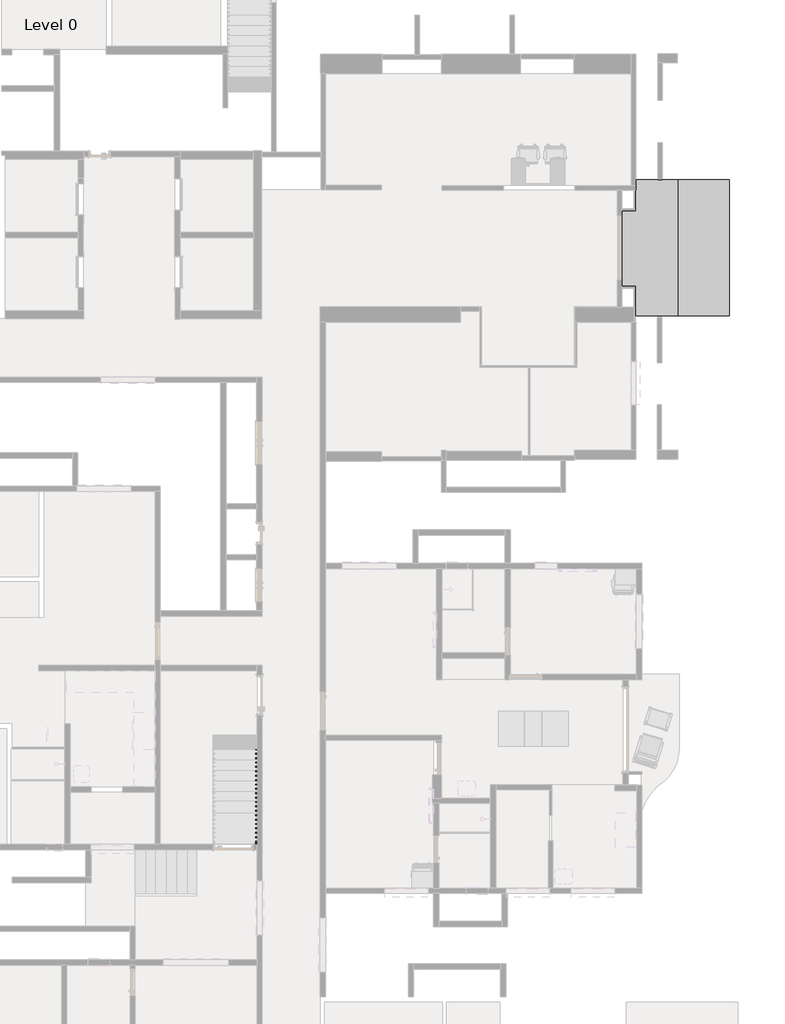
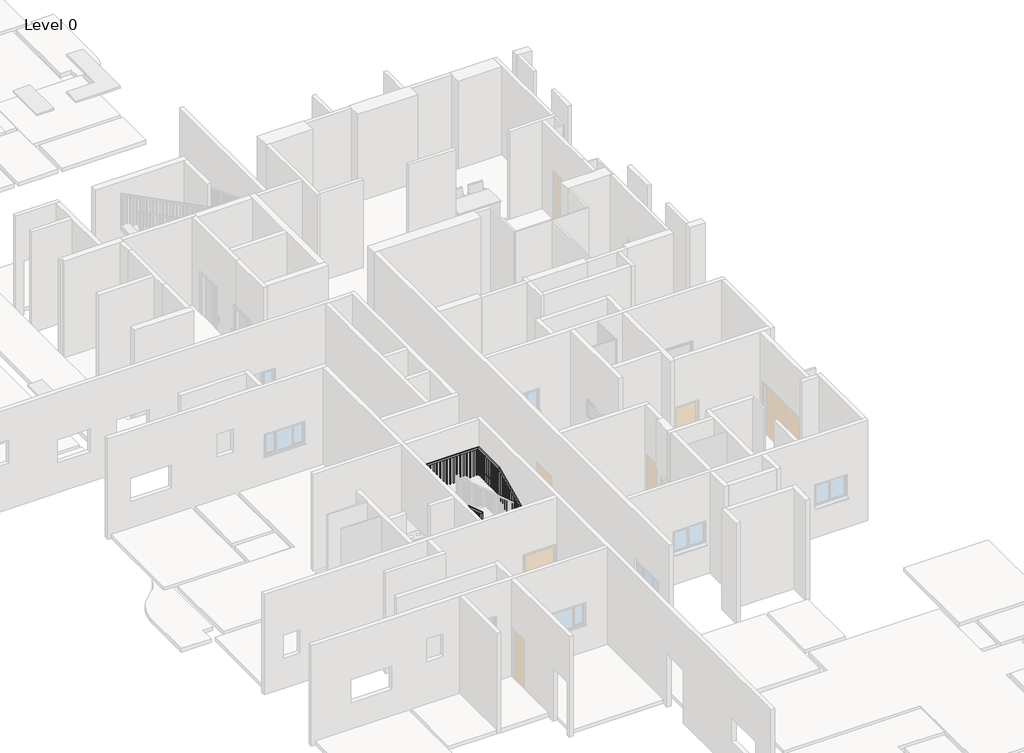
# One storey, part 11 of 14: 1 railing, 1 stair flight.
"""IFC4 building model written with IfcOpenShell, lengths in millimetres."""

from ifc_helpers import new_model, si_unit, frame, origin, place, context, project, spatial, polyline, outline, extrude, faceted_brep, element, save

model = new_model("IFC4")

# Units and contexts
model_context = context("Model", 3, world=origin())
ifc_project = project(units=[si_unit("LENGTHUNIT", "METRE", prefix="MILLI")], contexts=[model_context])

# Site, building, storey
site = spatial("IfcSite", under=ifc_project)
building = spatial("IfcBuilding", under=site)
storey = spatial("IfcBuildingStorey", under=building, Name="Level 0", Elevation=0.0)

# Railing
placement = place(None, origin())
element("IfcRailing", 1, ObjectType="1100mm", at=placement, inside=storey, context=model_context, shape_type="SolidModel", body=[
    faceted_brep([(-21794.7547508, 25955.1270746, 1266.6666667), (-21794.7547508, 25955.1270746, 1211.4472941), (-21744.7547508, 25955.1270746, 1211.4472941), (-21744.7547508, 25955.1270746, 1266.6666667), (-21794.7547508, 29511.1270746, 2933.3333333), (-21794.7547508, 29522.2631279, 2883.3333333), (-21744.7547508, 29522.2631279, 2883.3333333), (-21744.7547508, 29511.1270746, 2933.3333333), (-21794.7547508, 30833.6294818, 2933.3333333), (-21794.7547508, 30833.6294818, 2883.3333333), (-21744.7547508, 30883.6294818, 2883.3333333), (-21744.7547508, 30883.6294818, 2933.3333333), (-24444.1800447, 30833.6294818, 2933.3333333), (-24444.1800447, 30833.6294818, 2883.3333333), (-24494.1800447, 30883.6294818, 2883.3333333), (-24494.1800447, 30883.6294818, 2933.3333333), (-24444.1800447, 30021.9842175, 2933.3333333), (-24444.1800447, 30014.0341898, 2883.3333333), (-24494.1800447, 30014.0341898, 2883.3333333), (-24494.1800447, 30021.9842175, 2933.3333333), (-24444.1800447, 25935.1270746, 4266.6666667), (-24494.1800447, 25935.1270746, 4266.6666667), (-24494.1800447, 25935.1270746, 4214.0729775), (-24444.1800447, 25935.1270746, 4214.0729775)], [[[0, 1, 2, 3]], [[1, 0, 4, 5]], [[2, 1, 5, 6]], [[3, 2, 6, 7]], [[0, 3, 7, 4]], [[5, 4, 8, 9]], [[6, 5, 9, 10]], [[7, 6, 10, 11]], [[4, 7, 11, 8]], [[9, 8, 12, 13]], [[10, 9, 13, 14]], [[11, 10, 14, 15]], [[8, 11, 15, 12]], [[13, 12, 16, 17]], [[14, 13, 17, 18]], [[15, 14, 18, 19]], [[12, 15, 19, 16]], [[20, 21, 22, 23]], [[17, 16, 20, 23]], [[18, 17, 23, 22]], [[19, 18, 22, 21]], [[16, 19, 21, 20]]]),
    extrude(outline(polyline([(26058.6294818, 4173.7804323), (26058.6294818, 3000.0), (26033.6294818, 3000.0), (26033.6294818, 4181.936659), (26058.6294818, 4173.7804323)])), frame((-24481.6800447, 0.0, 0.0), z_axis=(1.0, 0.0, 0.0), x_axis=(0.0, 1.0, 0.0)), (0.0, 0.0, 1.0), 25.0),
    extrude(outline(polyline([(26183.6294818, 4132.9992988), (26183.6294818, 3000.0), (26158.6294818, 3000.0), (26158.6294818, 4141.1555255), (26183.6294818, 4132.9992988)])), frame((-24481.6800447, 0.0, 0.0), z_axis=(1.0, 0.0, 0.0), x_axis=(0.0, 1.0, 0.0)), (0.0, 0.0, 1.0), 25.0),
    extrude(outline(polyline([(26308.6294818, 4092.2181654), (26308.6294818, 3000.0), (26283.6294818, 3000.0), (26283.6294818, 4100.374392), (26308.6294818, 4092.2181654)])), frame((-24481.6800447, 0.0, 0.0), z_axis=(1.0, 0.0, 0.0), x_axis=(0.0, 1.0, 0.0)), (0.0, 0.0, 1.0), 25.0),
    extrude(outline(polyline([(26433.6294818, 4051.4370319), (26433.6294818, 3000.0), (26408.6294818, 3000.0), (26408.6294818, 4059.5932586), (26433.6294818, 4051.4370319)])), frame((-24481.6800447, 0.0, 0.0), z_axis=(1.0, 0.0, 0.0), x_axis=(0.0, 1.0, 0.0)), (0.0, 0.0, 1.0), 25.0),
    extrude(outline(polyline([(26558.6294818, 4010.6558984), (26558.6294818, 3000.0), (26533.6294818, 3000.0), (26533.6294818, 4018.8121251), (26558.6294818, 4010.6558984)])), frame((-24481.6800447, 0.0, 0.0), z_axis=(1.0, 0.0, 0.0), x_axis=(0.0, 1.0, 0.0)), (0.0, 0.0, 1.0), 25.0),
    extrude(outline(polyline([(26683.6294818, 3969.8747649), (26683.6294818, 3000.0), (26658.6294818, 3000.0), (26658.6294818, 3978.0309916), (26683.6294818, 3969.8747649)])), frame((-24481.6800447, 0.0, 0.0), z_axis=(1.0, 0.0, 0.0), x_axis=(0.0, 1.0, 0.0)), (0.0, 0.0, 1.0), 25.0),
    extrude(outline(polyline([(26808.6294818, 3929.0936314), (26808.6294818, 3000.0), (26783.6294818, 3000.0), (26783.6294818, 3937.2498581), (26808.6294818, 3929.0936314)])), frame((-24481.6800447, 0.0, 0.0), z_axis=(1.0, 0.0, 0.0), x_axis=(0.0, 1.0, 0.0)), (0.0, 0.0, 1.0), 25.0),
    extrude(outline(polyline([(26933.6294818, 3888.3124979), (26933.6294818, 3000.0), (26908.6294818, 3000.0), (26908.6294818, 3896.4687246), (26933.6294818, 3888.3124979)])), frame((-24481.6800447, 0.0, 0.0), z_axis=(1.0, 0.0, 0.0), x_axis=(0.0, 1.0, 0.0)), (0.0, 0.0, 1.0), 25.0),
    extrude(outline(polyline([(27058.6294818, 3847.5313645), (27058.6294818, 3000.0), (27033.6294818, 3000.0), (27033.6294818, 3855.6875912), (27058.6294818, 3847.5313645)])), frame((-24481.6800447, 0.0, 0.0), z_axis=(1.0, 0.0, 0.0), x_axis=(0.0, 1.0, 0.0)), (0.0, 0.0, 1.0), 25.0),
    extrude(outline(polyline([(27183.6294818, 3806.750231), (27183.6294818, 3000.0), (27158.6294818, 3000.0), (27158.6294818, 3814.9064577), (27183.6294818, 3806.750231)])), frame((-24481.6800447, 0.0, 0.0), z_axis=(1.0, 0.0, 0.0), x_axis=(0.0, 1.0, 0.0)), (0.0, 0.0, 1.0), 25.0),
    extrude(outline(polyline([(27308.6294818, 3765.9690975), (27308.6294818, 3000.0), (27283.6294818, 3000.0), (27283.6294818, 3774.1253242), (27308.6294818, 3765.9690975)])), frame((-24481.6800447, 0.0, 0.0), z_axis=(1.0, 0.0, 0.0), x_axis=(0.0, 1.0, 0.0)), (0.0, 0.0, 1.0), 25.0),
    extrude(outline(polyline([(27433.6294818, 3725.187964), (27433.6294818, 3000.0), (27408.6294818, 3000.0), (27408.6294818, 3733.3441907), (27433.6294818, 3725.187964)])), frame((-24481.6800447, 0.0, 0.0), z_axis=(1.0, 0.0, 0.0), x_axis=(0.0, 1.0, 0.0)), (0.0, 0.0, 1.0), 25.0),
    extrude(outline(polyline([(27558.6294818, 3684.4068305), (27558.6294818, 3000.0), (27533.6294818, 3000.0), (27533.6294818, 3692.5630572), (27558.6294818, 3684.4068305)])), frame((-24481.6800447, 0.0, 0.0), z_axis=(1.0, 0.0, 0.0), x_axis=(0.0, 1.0, 0.0)), (0.0, 0.0, 1.0), 25.0),
    extrude(outline(polyline([(27683.6294818, 3643.625697), (27683.6294818, 3000.0), (27658.6294818, 3000.0), (27658.6294818, 3651.7819237), (27683.6294818, 3643.625697)])), frame((-24481.6800447, 0.0, 0.0), z_axis=(1.0, 0.0, 0.0), x_axis=(0.0, 1.0, 0.0)), (0.0, 0.0, 1.0), 25.0),
    extrude(outline(polyline([(27808.6294818, 3602.8445636), (27808.6294818, 2833.3333333), (27783.6294818, 2833.3333333), (27783.6294818, 3611.0007903), (27808.6294818, 3602.8445636)])), frame((-24481.6800447, 0.0, 0.0), z_axis=(1.0, 0.0, 0.0), x_axis=(0.0, 1.0, 0.0)), (0.0, 0.0, 1.0), 25.0),
    extrude(outline(polyline([(27933.6294818, 3562.0634301), (27933.6294818, 2833.3333333), (27908.6294818, 2833.3333333), (27908.6294818, 3570.2196568), (27933.6294818, 3562.0634301)])), frame((-24481.6800447, 0.0, 0.0), z_axis=(1.0, 0.0, 0.0), x_axis=(0.0, 1.0, 0.0)), (0.0, 0.0, 1.0), 25.0),
    extrude(outline(polyline([(28058.6294818, 3521.2822966), (28058.6294818, 2833.3333333), (28033.6294818, 2833.3333333), (28033.6294818, 3529.4385233), (28058.6294818, 3521.2822966)])), frame((-24481.6800447, 0.0, 0.0), z_axis=(1.0, 0.0, 0.0), x_axis=(0.0, 1.0, 0.0)), (0.0, 0.0, 1.0), 25.0),
    extrude(outline(polyline([(28183.6294818, 3480.5011631), (28183.6294818, 2666.6666667), (28158.6294818, 2666.6666667), (28158.6294818, 3488.6573898), (28183.6294818, 3480.5011631)])), frame((-24481.6800447, 0.0, 0.0), z_axis=(1.0, 0.0, 0.0), x_axis=(0.0, 1.0, 0.0)), (0.0, 0.0, 1.0), 25.0),
    extrude(outline(polyline([(28308.6294818, 3439.7200296), (28308.6294818, 2666.6666667), (28283.6294818, 2666.6666667), (28283.6294818, 3447.8762563), (28308.6294818, 3439.7200296)])), frame((-24481.6800447, 0.0, 0.0), z_axis=(1.0, 0.0, 0.0), x_axis=(0.0, 1.0, 0.0)), (0.0, 0.0, 1.0), 25.0),
    extrude(outline(polyline([(28433.6294818, 3398.9388962), (28433.6294818, 2500.0), (28408.6294818, 2500.0), (28408.6294818, 3407.0951228), (28433.6294818, 3398.9388962)])), frame((-24481.6800447, 0.0, 0.0), z_axis=(1.0, 0.0, 0.0), x_axis=(0.0, 1.0, 0.0)), (0.0, 0.0, 1.0), 25.0),
    extrude(outline(polyline([(28558.6294818, 3358.1577627), (28558.6294818, 2500.0), (28533.6294818, 2500.0), (28533.6294818, 3366.3139894), (28558.6294818, 3358.1577627)])), frame((-24481.6800447, 0.0, 0.0), z_axis=(1.0, 0.0, 0.0), x_axis=(0.0, 1.0, 0.0)), (0.0, 0.0, 1.0), 25.0),
    extrude(outline(polyline([(28683.6294818, 3317.3766292), (28683.6294818, 2333.3333333), (28658.6294818, 2333.3333333), (28658.6294818, 3325.5328559), (28683.6294818, 3317.3766292)])), frame((-24481.6800447, 0.0, 0.0), z_axis=(1.0, 0.0, 0.0), x_axis=(0.0, 1.0, 0.0)), (0.0, 0.0, 1.0), 25.0),
    extrude(outline(polyline([(28808.6294818, 3276.5954957), (28808.6294818, 2333.3333333), (28783.6294818, 2333.3333333), (28783.6294818, 3284.7517224), (28808.6294818, 3276.5954957)])), frame((-24481.6800447, 0.0, 0.0), z_axis=(1.0, 0.0, 0.0), x_axis=(0.0, 1.0, 0.0)), (0.0, 0.0, 1.0), 25.0),
    extrude(outline(polyline([(28933.6294818, 3235.8143622), (28933.6294818, 2333.3333333), (28908.6294818, 2333.3333333), (28908.6294818, 3243.9705889), (28933.6294818, 3235.8143622)])), frame((-24481.6800447, 0.0, 0.0), z_axis=(1.0, 0.0, 0.0), x_axis=(0.0, 1.0, 0.0)), (0.0, 0.0, 1.0), 25.0),
    extrude(outline(polyline([(29058.6294818, 3195.0332287), (29058.6294818, 2166.6666667), (29033.6294818, 2166.6666667), (29033.6294818, 3203.1894554), (29058.6294818, 3195.0332287)])), frame((-24481.6800447, 0.0, 0.0), z_axis=(1.0, 0.0, 0.0), x_axis=(0.0, 1.0, 0.0)), (0.0, 0.0, 1.0), 25.0),
    extrude(outline(polyline([(29183.6294818, 3154.2520953), (29183.6294818, 2166.6666667), (29158.6294818, 2166.6666667), (29158.6294818, 3162.408322), (29183.6294818, 3154.2520953)])), frame((-24481.6800447, 0.0, 0.0), z_axis=(1.0, 0.0, 0.0), x_axis=(0.0, 1.0, 0.0)), (0.0, 0.0, 1.0), 25.0),
    extrude(outline(polyline([(29308.6294818, 3113.4709618), (29308.6294818, 2000.0), (29283.6294818, 2000.0), (29283.6294818, 3121.6271885), (29308.6294818, 3113.4709618)])), frame((-24481.6800447, 0.0, 0.0), z_axis=(1.0, 0.0, 0.0), x_axis=(0.0, 1.0, 0.0)), (0.0, 0.0, 1.0), 25.0),
    extrude(outline(polyline([(29433.6294818, 3072.6898283), (29433.6294818, 2000.0), (29408.6294818, 2000.0), (29408.6294818, 3080.846055), (29433.6294818, 3072.6898283)])), frame((-24481.6800447, 0.0, 0.0), z_axis=(1.0, 0.0, 0.0), x_axis=(0.0, 1.0, 0.0)), (0.0, 0.0, 1.0), 25.0),
    extrude(outline(polyline([(29558.6294818, 3031.9086948), (29558.6294818, 1833.3333333), (29533.6294818, 1833.3333333), (29533.6294818, 3040.0649215), (29558.6294818, 3031.9086948)])), frame((-24481.6800447, 0.0, 0.0), z_axis=(1.0, 0.0, 0.0), x_axis=(0.0, 1.0, 0.0)), (0.0, 0.0, 1.0), 25.0),
    extrude(outline(polyline([(29683.6294818, 2991.1275613), (29683.6294818, 1833.3333333), (29658.6294818, 1833.3333333), (29658.6294818, 2999.283788), (29683.6294818, 2991.1275613)])), frame((-24481.6800447, 0.0, 0.0), z_axis=(1.0, 0.0, 0.0), x_axis=(0.0, 1.0, 0.0)), (0.0, 0.0, 1.0), 25.0),
    extrude(outline(polyline([(29808.6294818, 2950.3464278), (29808.6294818, 1833.3333333), (29783.6294818, 1833.3333333), (29783.6294818, 2958.5026545), (29808.6294818, 2950.3464278)])), frame((-24481.6800447, 0.0, 0.0), z_axis=(1.0, 0.0, 0.0), x_axis=(0.0, 1.0, 0.0)), (0.0, 0.0, 1.0), 25.0),
    extrude(outline(polyline([(29933.6294818, 2909.5652944), (29933.6294818, 1833.3333333), (29908.6294818, 1833.3333333), (29908.6294818, 2917.7215211), (29933.6294818, 2909.5652944)])), frame((-24481.6800447, 0.0, 0.0), z_axis=(1.0, 0.0, 0.0), x_axis=(0.0, 1.0, 0.0)), (0.0, 0.0, 1.0), 25.0),
    extrude(outline(polyline([(-24481.6800447, 30058.6294818), (-24456.6800447, 30058.6294818), (-24456.6800447, 30033.6294818), (-24481.6800447, 30033.6294818), (-24481.6800447, 30058.6294818)])), frame((0.0, 0.0, 1833.3333333), z_axis=(0.0, 0.0, 1.0), x_axis=(1.0, 0.0, 0.0)), (0.0, 0.0, 1.0), 1050.0),
    extrude(outline(polyline([(-24481.6800447, 30183.6294818), (-24456.6800447, 30183.6294818), (-24456.6800447, 30158.6294818), (-24481.6800447, 30158.6294818), (-24481.6800447, 30183.6294818)])), frame((0.0, 0.0, 1833.3333333), z_axis=(0.0, 0.0, 1.0), x_axis=(1.0, 0.0, 0.0)), (0.0, 0.0, 1.0), 1050.0),
    extrude(outline(polyline([(-24481.6800447, 30308.6294818), (-24456.6800447, 30308.6294818), (-24456.6800447, 30283.6294818), (-24481.6800447, 30283.6294818), (-24481.6800447, 30308.6294818)])), frame((0.0, 0.0, 1833.3333333), z_axis=(0.0, 0.0, 1.0), x_axis=(1.0, 0.0, 0.0)), (0.0, 0.0, 1.0), 1050.0),
    extrude(outline(polyline([(-24481.6800447, 30433.6294818), (-24456.6800447, 30433.6294818), (-24456.6800447, 30408.6294818), (-24481.6800447, 30408.6294818), (-24481.6800447, 30433.6294818)])), frame((0.0, 0.0, 1833.3333333), z_axis=(0.0, 0.0, 1.0), x_axis=(1.0, 0.0, 0.0)), (0.0, 0.0, 1.0), 1050.0),
    extrude(outline(polyline([(-24481.6800447, 30558.6294818), (-24456.6800447, 30558.6294818), (-24456.6800447, 30533.6294818), (-24481.6800447, 30533.6294818), (-24481.6800447, 30558.6294818)])), frame((0.0, 0.0, 1833.3333333), z_axis=(0.0, 0.0, 1.0), x_axis=(1.0, 0.0, 0.0)), (0.0, 0.0, 1.0), 1050.0),
    extrude(outline(polyline([(-24481.6800447, 30683.6294818), (-24456.6800447, 30683.6294818), (-24456.6800447, 30658.6294818), (-24481.6800447, 30658.6294818), (-24481.6800447, 30683.6294818)])), frame((0.0, 0.0, 1833.3333333), z_axis=(0.0, 0.0, 1.0), x_axis=(1.0, 0.0, 0.0)), (0.0, 0.0, 1.0), 1050.0),
    extrude(outline(polyline([(-24481.6800447, 30808.6294818), (-24456.6800447, 30808.6294818), (-24456.6800447, 30783.6294818), (-24481.6800447, 30783.6294818), (-24481.6800447, 30808.6294818)])), frame((0.0, 0.0, 1833.3333333), z_axis=(0.0, 0.0, 1.0), x_axis=(1.0, 0.0, 0.0)), (0.0, 0.0, 1.0), 1050.0),
    extrude(outline(polyline([(-24444.7547508, 30871.1294818), (-24444.7547508, 30846.1294818), (-24469.7547508, 30846.1294818), (-24469.7547508, 30871.1294818), (-24444.7547508, 30871.1294818)])), frame((0.0, 0.0, 1833.3333333), z_axis=(0.0, 0.0, 1.0), x_axis=(1.0, 0.0, 0.0)), (0.0, 0.0, 1.0), 1050.0),
    extrude(outline(polyline([(-24319.7547508, 30871.1294818), (-24319.7547508, 30846.1294818), (-24344.7547508, 30846.1294818), (-24344.7547508, 30871.1294818), (-24319.7547508, 30871.1294818)])), frame((0.0, 0.0, 1833.3333333), z_axis=(0.0, 0.0, 1.0), x_axis=(1.0, 0.0, 0.0)), (0.0, 0.0, 1.0), 1050.0),
    extrude(outline(polyline([(-24194.7547508, 30871.1294818), (-24194.7547508, 30846.1294818), (-24219.7547508, 30846.1294818), (-24219.7547508, 30871.1294818), (-24194.7547508, 30871.1294818)])), frame((0.0, 0.0, 1833.3333333), z_axis=(0.0, 0.0, 1.0), x_axis=(1.0, 0.0, 0.0)), (0.0, 0.0, 1.0), 1050.0),
    extrude(outline(polyline([(-24069.7547508, 30871.1294818), (-24069.7547508, 30846.1294818), (-24094.7547508, 30846.1294818), (-24094.7547508, 30871.1294818), (-24069.7547508, 30871.1294818)])), frame((0.0, 0.0, 1833.3333333), z_axis=(0.0, 0.0, 1.0), x_axis=(1.0, 0.0, 0.0)), (0.0, 0.0, 1.0), 1050.0),
    extrude(outline(polyline([(-23944.7547508, 30871.1294818), (-23944.7547508, 30846.1294818), (-23969.7547508, 30846.1294818), (-23969.7547508, 30871.1294818), (-23944.7547508, 30871.1294818)])), frame((0.0, 0.0, 1833.3333333), z_axis=(0.0, 0.0, 1.0), x_axis=(1.0, 0.0, 0.0)), (0.0, 0.0, 1.0), 1050.0),
    extrude(outline(polyline([(-23819.7547508, 30871.1294818), (-23819.7547508, 30846.1294818), (-23844.7547508, 30846.1294818), (-23844.7547508, 30871.1294818), (-23819.7547508, 30871.1294818)])), frame((0.0, 0.0, 1833.3333333), z_axis=(0.0, 0.0, 1.0), x_axis=(1.0, 0.0, 0.0)), (0.0, 0.0, 1.0), 1050.0),
    extrude(outline(polyline([(-23694.7547508, 30871.1294818), (-23694.7547508, 30846.1294818), (-23719.7547508, 30846.1294818), (-23719.7547508, 30871.1294818), (-23694.7547508, 30871.1294818)])), frame((0.0, 0.0, 1833.3333333), z_axis=(0.0, 0.0, 1.0), x_axis=(1.0, 0.0, 0.0)), (0.0, 0.0, 1.0), 1050.0),
    extrude(outline(polyline([(-23569.7547508, 30871.1294818), (-23569.7547508, 30846.1294818), (-23594.7547508, 30846.1294818), (-23594.7547508, 30871.1294818), (-23569.7547508, 30871.1294818)])), frame((0.0, 0.0, 1833.3333333), z_axis=(0.0, 0.0, 1.0), x_axis=(1.0, 0.0, 0.0)), (0.0, 0.0, 1.0), 1050.0),
    extrude(outline(polyline([(-23444.7547508, 30871.1294818), (-23444.7547508, 30846.1294818), (-23469.7547508, 30846.1294818), (-23469.7547508, 30871.1294818), (-23444.7547508, 30871.1294818)])), frame((0.0, 0.0, 1833.3333333), z_axis=(0.0, 0.0, 1.0), x_axis=(1.0, 0.0, 0.0)), (0.0, 0.0, 1.0), 1050.0),
    extrude(outline(polyline([(-23319.7547508, 30871.1294818), (-23319.7547508, 30846.1294818), (-23344.7547508, 30846.1294818), (-23344.7547508, 30871.1294818), (-23319.7547508, 30871.1294818)])), frame((0.0, 0.0, 1833.3333333), z_axis=(0.0, 0.0, 1.0), x_axis=(1.0, 0.0, 0.0)), (0.0, 0.0, 1.0), 1050.0),
    extrude(outline(polyline([(-23194.7547508, 30871.1294818), (-23194.7547508, 30846.1294818), (-23219.7547508, 30846.1294818), (-23219.7547508, 30871.1294818), (-23194.7547508, 30871.1294818)])), frame((0.0, 0.0, 1833.3333333), z_axis=(0.0, 0.0, 1.0), x_axis=(1.0, 0.0, 0.0)), (0.0, 0.0, 1.0), 1050.0),
    extrude(outline(polyline([(-23069.7547508, 30871.1294818), (-23069.7547508, 30846.1294818), (-23094.7547508, 30846.1294818), (-23094.7547508, 30871.1294818), (-23069.7547508, 30871.1294818)])), frame((0.0, 0.0, 1833.3333333), z_axis=(0.0, 0.0, 1.0), x_axis=(1.0, 0.0, 0.0)), (0.0, 0.0, 1.0), 1050.0),
    extrude(outline(polyline([(-22944.7547508, 30871.1294818), (-22944.7547508, 30846.1294818), (-22969.7547508, 30846.1294818), (-22969.7547508, 30871.1294818), (-22944.7547508, 30871.1294818)])), frame((0.0, 0.0, 1833.3333333), z_axis=(0.0, 0.0, 1.0), x_axis=(1.0, 0.0, 0.0)), (0.0, 0.0, 1.0), 1050.0),
    extrude(outline(polyline([(-22819.7547508, 30871.1294818), (-22819.7547508, 30846.1294818), (-22844.7547508, 30846.1294818), (-22844.7547508, 30871.1294818), (-22819.7547508, 30871.1294818)])), frame((0.0, 0.0, 1833.3333333), z_axis=(0.0, 0.0, 1.0), x_axis=(1.0, 0.0, 0.0)), (0.0, 0.0, 1.0), 1050.0),
    extrude(outline(polyline([(-22694.7547508, 30871.1294818), (-22694.7547508, 30846.1294818), (-22719.7547508, 30846.1294818), (-22719.7547508, 30871.1294818), (-22694.7547508, 30871.1294818)])), frame((0.0, 0.0, 1833.3333333), z_axis=(0.0, 0.0, 1.0), x_axis=(1.0, 0.0, 0.0)), (0.0, 0.0, 1.0), 1050.0),
    extrude(outline(polyline([(-22569.7547508, 30871.1294818), (-22569.7547508, 30846.1294818), (-22594.7547508, 30846.1294818), (-22594.7547508, 30871.1294818), (-22569.7547508, 30871.1294818)])), frame((0.0, 0.0, 1833.3333333), z_axis=(0.0, 0.0, 1.0), x_axis=(1.0, 0.0, 0.0)), (0.0, 0.0, 1.0), 1050.0),
    extrude(outline(polyline([(-22444.7547508, 30871.1294818), (-22444.7547508, 30846.1294818), (-22469.7547508, 30846.1294818), (-22469.7547508, 30871.1294818), (-22444.7547508, 30871.1294818)])), frame((0.0, 0.0, 1833.3333333), z_axis=(0.0, 0.0, 1.0), x_axis=(1.0, 0.0, 0.0)), (0.0, 0.0, 1.0), 1050.0),
    extrude(outline(polyline([(-22319.7547508, 30871.1294818), (-22319.7547508, 30846.1294818), (-22344.7547508, 30846.1294818), (-22344.7547508, 30871.1294818), (-22319.7547508, 30871.1294818)])), frame((0.0, 0.0, 1833.3333333), z_axis=(0.0, 0.0, 1.0), x_axis=(1.0, 0.0, 0.0)), (0.0, 0.0, 1.0), 1050.0),
    extrude(outline(polyline([(-22194.7547508, 30871.1294818), (-22194.7547508, 30846.1294818), (-22219.7547508, 30846.1294818), (-22219.7547508, 30871.1294818), (-22194.7547508, 30871.1294818)])), frame((0.0, 0.0, 1833.3333333), z_axis=(0.0, 0.0, 1.0), x_axis=(1.0, 0.0, 0.0)), (0.0, 0.0, 1.0), 1050.0),
    extrude(outline(polyline([(-22069.7547508, 30871.1294818), (-22069.7547508, 30846.1294818), (-22094.7547508, 30846.1294818), (-22094.7547508, 30871.1294818), (-22069.7547508, 30871.1294818)])), frame((0.0, 0.0, 1833.3333333), z_axis=(0.0, 0.0, 1.0), x_axis=(1.0, 0.0, 0.0)), (0.0, 0.0, 1.0), 1050.0),
    extrude(outline(polyline([(-21944.7547508, 30871.1294818), (-21944.7547508, 30846.1294818), (-21969.7547508, 30846.1294818), (-21969.7547508, 30871.1294818), (-21944.7547508, 30871.1294818)])), frame((0.0, 0.0, 1833.3333333), z_axis=(0.0, 0.0, 1.0), x_axis=(1.0, 0.0, 0.0)), (0.0, 0.0, 1.0), 1050.0),
    extrude(outline(polyline([(-21819.7547508, 30871.1294818), (-21819.7547508, 30846.1294818), (-21844.7547508, 30846.1294818), (-21844.7547508, 30871.1294818), (-21819.7547508, 30871.1294818)])), frame((0.0, 0.0, 1833.3333333), z_axis=(0.0, 0.0, 1.0), x_axis=(1.0, 0.0, 0.0)), (0.0, 0.0, 1.0), 1050.0),
    extrude(outline(polyline([(-21757.2547508, 30755.1270746), (-21782.2547508, 30755.1270746), (-21782.2547508, 30780.1270746), (-21757.2547508, 30780.1270746), (-21757.2547508, 30755.1270746)])), frame((0.0, 0.0, 1833.3333333), z_axis=(0.0, 0.0, 1.0), x_axis=(1.0, 0.0, 0.0)), (0.0, 0.0, 1.0), 1050.0),
    extrude(outline(polyline([(-21757.2547508, 30630.1270746), (-21782.2547508, 30630.1270746), (-21782.2547508, 30655.1270746), (-21757.2547508, 30655.1270746), (-21757.2547508, 30630.1270746)])), frame((0.0, 0.0, 1833.3333333), z_axis=(0.0, 0.0, 1.0), x_axis=(1.0, 0.0, 0.0)), (0.0, 0.0, 1.0), 1050.0),
    extrude(outline(polyline([(-21757.2547508, 30505.1270746), (-21782.2547508, 30505.1270746), (-21782.2547508, 30530.1270746), (-21757.2547508, 30530.1270746), (-21757.2547508, 30505.1270746)])), frame((0.0, 0.0, 1833.3333333), z_axis=(0.0, 0.0, 1.0), x_axis=(1.0, 0.0, 0.0)), (0.0, 0.0, 1.0), 1050.0),
    extrude(outline(polyline([(-21757.2547508, 30380.1270746), (-21782.2547508, 30380.1270746), (-21782.2547508, 30405.1270746), (-21757.2547508, 30405.1270746), (-21757.2547508, 30380.1270746)])), frame((0.0, 0.0, 1833.3333333), z_axis=(0.0, 0.0, 1.0), x_axis=(1.0, 0.0, 0.0)), (0.0, 0.0, 1.0), 1050.0),
    extrude(outline(polyline([(-21757.2547508, 30255.1270746), (-21782.2547508, 30255.1270746), (-21782.2547508, 30280.1270746), (-21757.2547508, 30280.1270746), (-21757.2547508, 30255.1270746)])), frame((0.0, 0.0, 1833.3333333), z_axis=(0.0, 0.0, 1.0), x_axis=(1.0, 0.0, 0.0)), (0.0, 0.0, 1.0), 1050.0),
    extrude(outline(polyline([(-21757.2547508, 30130.1270746), (-21782.2547508, 30130.1270746), (-21782.2547508, 30155.1270746), (-21757.2547508, 30155.1270746), (-21757.2547508, 30130.1270746)])), frame((0.0, 0.0, 1833.3333333), z_axis=(0.0, 0.0, 1.0), x_axis=(1.0, 0.0, 0.0)), (0.0, 0.0, 1.0), 1050.0),
    extrude(outline(polyline([(-21757.2547508, 30005.1270746), (-21782.2547508, 30005.1270746), (-21782.2547508, 30030.1270746), (-21757.2547508, 30030.1270746), (-21757.2547508, 30005.1270746)])), frame((0.0, 0.0, 1833.3333333), z_axis=(0.0, 0.0, 1.0), x_axis=(1.0, 0.0, 0.0)), (0.0, 0.0, 1.0), 1050.0),
    extrude(outline(polyline([(-21757.2547508, 29880.1270746), (-21782.2547508, 29880.1270746), (-21782.2547508, 29905.1270746), (-21757.2547508, 29905.1270746), (-21757.2547508, 29880.1270746)])), frame((0.0, 0.0, 1833.3333333), z_axis=(0.0, 0.0, 1.0), x_axis=(1.0, 0.0, 0.0)), (0.0, 0.0, 1.0), 1050.0),
    extrude(outline(polyline([(-21757.2547508, 29755.1270746), (-21782.2547508, 29755.1270746), (-21782.2547508, 29780.1270746), (-21757.2547508, 29780.1270746), (-21757.2547508, 29755.1270746)])), frame((0.0, 0.0, 1833.3333333), z_axis=(0.0, 0.0, 1.0), x_axis=(1.0, 0.0, 0.0)), (0.0, 0.0, 1.0), 1050.0),
    extrude(outline(polyline([(-21757.2547508, 29630.1270746), (-21782.2547508, 29630.1270746), (-21782.2547508, 29655.1270746), (-21757.2547508, 29655.1270746), (-21757.2547508, 29630.1270746)])), frame((0.0, 0.0, 1833.3333333), z_axis=(0.0, 0.0, 1.0), x_axis=(1.0, 0.0, 0.0)), (0.0, 0.0, 1.0), 1050.0),
    extrude(outline(polyline([(-21757.2547508, 29505.1270746), (-21782.2547508, 29505.1270746), (-21782.2547508, 29530.1270746), (-21757.2547508, 29530.1270746), (-21757.2547508, 29505.1270746)])), frame((0.0, 0.0, 1833.3333333), z_axis=(0.0, 0.0, 1.0), x_axis=(1.0, 0.0, 0.0)), (0.0, 0.0, 1.0), 1050.0),
    extrude(outline(polyline([(29380.1270746, 1666.6666667), (29380.1270746, 2816.7153856), (29405.1270746, 2828.432671), (29405.1270746, 1666.6666667), (29380.1270746, 1666.6666667)])), frame((-21782.2547508, 0.0, 0.0), z_axis=(1.0, 0.0, 0.0), x_axis=(0.0, 1.0, 0.0)), (0.0, 0.0, 1.0), 25.0),
    extrude(outline(polyline([(29255.1270746, 1666.6666667), (29255.1270746, 2758.1289589), (29280.1270746, 2769.8462443), (29280.1270746, 1666.6666667), (29255.1270746, 1666.6666667)])), frame((-21782.2547508, 0.0, 0.0), z_axis=(1.0, 0.0, 0.0), x_axis=(0.0, 1.0, 0.0)), (0.0, 0.0, 1.0), 25.0),
    extrude(outline(polyline([(29130.1270746, 1500.0), (29130.1270746, 2699.5425322), (29155.1270746, 2711.2598176), (29155.1270746, 1500.0), (29130.1270746, 1500.0)])), frame((-21782.2547508, 0.0, 0.0), z_axis=(1.0, 0.0, 0.0), x_axis=(0.0, 1.0, 0.0)), (0.0, 0.0, 1.0), 25.0),
    extrude(outline(polyline([(29005.1270746, 1500.0), (29005.1270746, 2640.9561055), (29030.1270746, 2652.6733909), (29030.1270746, 1500.0), (29005.1270746, 1500.0)])), frame((-21782.2547508, 0.0, 0.0), z_axis=(1.0, 0.0, 0.0), x_axis=(0.0, 1.0, 0.0)), (0.0, 0.0, 1.0), 25.0),
    extrude(outline(polyline([(28880.1270746, 1333.3333333), (28880.1270746, 2582.3696788), (28905.1270746, 2594.0869642), (28905.1270746, 1333.3333333), (28880.1270746, 1333.3333333)])), frame((-21782.2547508, 0.0, 0.0), z_axis=(1.0, 0.0, 0.0), x_axis=(0.0, 1.0, 0.0)), (0.0, 0.0, 1.0), 25.0),
    extrude(outline(polyline([(28755.1270746, 1333.3333333), (28755.1270746, 2523.7832521), (28780.1270746, 2535.5005375), (28780.1270746, 1333.3333333), (28755.1270746, 1333.3333333)])), frame((-21782.2547508, 0.0, 0.0), z_axis=(1.0, 0.0, 0.0), x_axis=(0.0, 1.0, 0.0)), (0.0, 0.0, 1.0), 25.0),
    extrude(outline(polyline([(28630.1270746, 1166.6666667), (28630.1270746, 2465.1968254), (28655.1270746, 2476.9141108), (28655.1270746, 1166.6666667), (28630.1270746, 1166.6666667)])), frame((-21782.2547508, 0.0, 0.0), z_axis=(1.0, 0.0, 0.0), x_axis=(0.0, 1.0, 0.0)), (0.0, 0.0, 1.0), 25.0),
    extrude(outline(polyline([(28505.1270746, 1166.6666667), (28505.1270746, 2406.6103987), (28530.1270746, 2418.3276841), (28530.1270746, 1166.6666667), (28505.1270746, 1166.6666667)])), frame((-21782.2547508, 0.0, 0.0), z_axis=(1.0, 0.0, 0.0), x_axis=(0.0, 1.0, 0.0)), (0.0, 0.0, 1.0), 25.0),
    extrude(outline(polyline([(28380.1270746, 1166.6666667), (28380.1270746, 2348.023972), (28405.1270746, 2359.7412574), (28405.1270746, 1166.6666667), (28380.1270746, 1166.6666667)])), frame((-21782.2547508, 0.0, 0.0), z_axis=(1.0, 0.0, 0.0), x_axis=(0.0, 1.0, 0.0)), (0.0, 0.0, 1.0), 25.0),
    extrude(outline(polyline([(28255.1270746, 1000.0), (28255.1270746, 2289.4375454), (28280.1270746, 2301.1548307), (28280.1270746, 1000.0), (28255.1270746, 1000.0)])), frame((-21782.2547508, 0.0, 0.0), z_axis=(1.0, 0.0, 0.0), x_axis=(0.0, 1.0, 0.0)), (0.0, 0.0, 1.0), 25.0),
    extrude(outline(polyline([(28130.1270746, 1000.0), (28130.1270746, 2230.8511187), (28155.1270746, 2242.568404), (28155.1270746, 1000.0), (28130.1270746, 1000.0)])), frame((-21782.2547508, 0.0, 0.0), z_axis=(1.0, 0.0, 0.0), x_axis=(0.0, 1.0, 0.0)), (0.0, 0.0, 1.0), 25.0),
    extrude(outline(polyline([(28005.1270746, 833.3333333), (28005.1270746, 2172.264692), (28030.1270746, 2183.9819773), (28030.1270746, 833.3333333), (28005.1270746, 833.3333333)])), frame((-21782.2547508, 0.0, 0.0), z_axis=(1.0, 0.0, 0.0), x_axis=(0.0, 1.0, 0.0)), (0.0, 0.0, 1.0), 25.0),
    extrude(outline(polyline([(27880.1270746, 833.3333333), (27880.1270746, 2113.6782653), (27905.1270746, 2125.3955506), (27905.1270746, 833.3333333), (27880.1270746, 833.3333333)])), frame((-21782.2547508, 0.0, 0.0), z_axis=(1.0, 0.0, 0.0), x_axis=(0.0, 1.0, 0.0)), (0.0, 0.0, 1.0), 25.0),
    extrude(outline(polyline([(27755.1270746, 833.3333333), (27755.1270746, 2055.0918386), (27780.1270746, 2066.8091239), (27780.1270746, 833.3333333), (27755.1270746, 833.3333333)])), frame((-21782.2547508, 0.0, 0.0), z_axis=(1.0, 0.0, 0.0), x_axis=(0.0, 1.0, 0.0)), (0.0, 0.0, 1.0), 25.0),
    extrude(outline(polyline([(27630.1270746, 666.6666667), (27630.1270746, 1996.5054119), (27655.1270746, 2008.2226972), (27655.1270746, 666.6666667), (27630.1270746, 666.6666667)])), frame((-21782.2547508, 0.0, 0.0), z_axis=(1.0, 0.0, 0.0), x_axis=(0.0, 1.0, 0.0)), (0.0, 0.0, 1.0), 25.0),
    extrude(outline(polyline([(27505.1270746, 666.6666667), (27505.1270746, 1937.9189852), (27530.1270746, 1949.6362705), (27530.1270746, 666.6666667), (27505.1270746, 666.6666667)])), frame((-21782.2547508, 0.0, 0.0), z_axis=(1.0, 0.0, 0.0), x_axis=(0.0, 1.0, 0.0)), (0.0, 0.0, 1.0), 25.0),
    extrude(outline(polyline([(27380.1270746, 500.0), (27380.1270746, 1879.3325585), (27405.1270746, 1891.0498438), (27405.1270746, 500.0), (27380.1270746, 500.0)])), frame((-21782.2547508, 0.0, 0.0), z_axis=(1.0, 0.0, 0.0), x_axis=(0.0, 1.0, 0.0)), (0.0, 0.0, 1.0), 25.0),
    extrude(outline(polyline([(27255.1270746, 500.0), (27255.1270746, 1820.7461318), (27280.1270746, 1832.4634171), (27280.1270746, 500.0), (27255.1270746, 500.0)])), frame((-21782.2547508, 0.0, 0.0), z_axis=(1.0, 0.0, 0.0), x_axis=(0.0, 1.0, 0.0)), (0.0, 0.0, 1.0), 25.0),
    extrude(outline(polyline([(27130.1270746, 333.3333333), (27130.1270746, 1762.1597051), (27155.1270746, 1773.8769904), (27155.1270746, 333.3333333), (27130.1270746, 333.3333333)])), frame((-21782.2547508, 0.0, 0.0), z_axis=(1.0, 0.0, 0.0), x_axis=(0.0, 1.0, 0.0)), (0.0, 0.0, 1.0), 25.0),
    extrude(outline(polyline([(27005.1270746, 333.3333333), (27005.1270746, 1703.5732784), (27030.1270746, 1715.2905637), (27030.1270746, 333.3333333), (27005.1270746, 333.3333333)])), frame((-21782.2547508, 0.0, 0.0), z_axis=(1.0, 0.0, 0.0), x_axis=(0.0, 1.0, 0.0)), (0.0, 0.0, 1.0), 25.0),
    extrude(outline(polyline([(26880.1270746, 333.3333333), (26880.1270746, 1644.9868517), (26905.1270746, 1656.704137), (26905.1270746, 333.3333333), (26880.1270746, 333.3333333)])), frame((-21782.2547508, 0.0, 0.0), z_axis=(1.0, 0.0, 0.0), x_axis=(0.0, 1.0, 0.0)), (0.0, 0.0, 1.0), 25.0),
    extrude(outline(polyline([(26755.1270746, 166.6666667), (26755.1270746, 1586.400425), (26780.1270746, 1598.1177103), (26780.1270746, 166.6666667), (26755.1270746, 166.6666667)])), frame((-21782.2547508, 0.0, 0.0), z_axis=(1.0, 0.0, 0.0), x_axis=(0.0, 1.0, 0.0)), (0.0, 0.0, 1.0), 25.0),
    extrude(outline(polyline([(26630.1270746, 166.6666667), (26630.1270746, 1527.8139983), (26655.1270746, 1539.5312836), (26655.1270746, 166.6666667), (26630.1270746, 166.6666667)])), frame((-21782.2547508, 0.0, 0.0), z_axis=(1.0, 0.0, 0.0), x_axis=(0.0, 1.0, 0.0)), (0.0, 0.0, 1.0), 25.0),
    extrude(outline(polyline([(26505.1270746, 166.6666667), (26505.1270746, 1469.2275716), (26530.1270746, 1480.9448569), (26530.1270746, 166.6666667), (26505.1270746, 166.6666667)])), frame((-21782.2547508, 0.0, 0.0), z_axis=(1.0, 0.0, 0.0), x_axis=(0.0, 1.0, 0.0)), (0.0, 0.0, 1.0), 25.0),
    extrude(outline(polyline([(26380.1270746, 166.6666667), (26380.1270746, 1410.6411449), (26405.1270746, 1422.3584302), (26405.1270746, 166.6666667), (26380.1270746, 166.6666667)])), frame((-21782.2547508, 0.0, 0.0), z_axis=(1.0, 0.0, 0.0), x_axis=(0.0, 1.0, 0.0)), (0.0, 0.0, 1.0), 25.0),
    extrude(outline(polyline([(26255.1270746, 166.6666667), (26255.1270746, 1352.0547182), (26280.1270746, 1363.7720035), (26280.1270746, 166.6666667), (26255.1270746, 166.6666667)])), frame((-21782.2547508, 0.0, 0.0), z_axis=(1.0, 0.0, 0.0), x_axis=(0.0, 1.0, 0.0)), (0.0, 0.0, 1.0), 25.0),
    extrude(outline(polyline([(26130.1270746, 166.6666667), (26130.1270746, 1293.4682915), (26155.1270746, 1305.1855768), (26155.1270746, 166.6666667), (26130.1270746, 166.6666667)])), frame((-21782.2547508, 0.0, 0.0), z_axis=(1.0, 0.0, 0.0), x_axis=(0.0, 1.0, 0.0)), (0.0, 0.0, 1.0), 25.0),
    extrude(outline(polyline([(26005.1270746, 166.6666667), (26005.1270746, 1234.8818648), (26030.1270746, 1246.5991502), (26030.1270746, 166.6666667), (26005.1270746, 166.6666667)])), frame((-21782.2547508, 0.0, 0.0), z_axis=(1.0, 0.0, 0.0), x_axis=(0.0, 1.0, 0.0)), (0.0, 0.0, 1.0), 25.0),
    extrude(outline(polyline([(-24456.6800447, 30871.1294818), (-24456.6800447, 30846.1294818), (-24481.6800447, 30846.1294818), (-24481.6800447, 30871.1294818), (-24456.6800447, 30871.1294818)])), frame((0.0, 0.0, 1833.3333333), z_axis=(0.0, 0.0, 1.0), x_axis=(1.0, 0.0, 0.0)), (0.0, 0.0, 1.0), 1050.0),
    extrude(outline(polyline([(-21757.2547508, 30846.1294818), (-21782.2547508, 30846.1294818), (-21782.2547508, 30871.1294818), (-21757.2547508, 30871.1294818), (-21757.2547508, 30846.1294818)])), frame((0.0, 0.0, 1833.3333333), z_axis=(0.0, 0.0, 1.0), x_axis=(1.0, 0.0, 0.0)), (0.0, 0.0, 1.0), 1050.0),
    extrude(outline(polyline([(25960.1270746, 4205.9167508), (25960.1270746, 3000.0), (25935.1270746, 3000.0), (25935.1270746, 4214.0729775), (25960.1270746, 4205.9167508)])), frame((-24481.6800447, 0.0, 0.0), z_axis=(1.0, 0.0, 0.0), x_axis=(0.0, 1.0, 0.0)), (0.0, 0.0, 1.0), 25.0),
    extrude(outline(polyline([(25955.1270746, 166.6666667), (25955.1270746, 1211.4472941), (25980.1270746, 1223.1645795), (25980.1270746, 166.6666667), (25955.1270746, 166.6666667)])), frame((-21782.2547508, 0.0, 0.0), z_axis=(1.0, 0.0, 0.0), x_axis=(0.0, 1.0, 0.0)), (0.0, 0.0, 1.0), 25.0),
])

# Stair flight
element("IfcStairFlight", 2, ObjectType="1mm_Tread-175mm_Depth", at=placement, inside=storey, context=model_context, shape_type="SolidModel", body=[
    faceted_brep([(-9747.8226051, 40981.3652361, 165.6666667), (-8281.7950217, 40981.3652361, 165.6666667), (-8281.7950217, 44862.7031635, 165.6666667), (-9747.8226051, 44862.7031635, 165.6666667), (-9747.8226051, 40981.3652361, 157.3333333), (-9747.8226051, 40981.3652361, 0.0), (-8281.7950217, 40981.3652361, 0.0), (-8281.7950217, 44862.7031635, 0.0), (-9747.8226051, 44862.7031635, 0.0), (-9747.8226051, 44862.7031635, 157.3333333), (-11329.7950217, 41844.9652361, 332.3333333), (-10948.7950217, 41844.9652361, 332.3333333), (-10948.7950217, 40981.3652361, 332.3333333), (-9747.8226051, 40981.3652361, 332.3333333), (-9747.8226051, 44862.7031635, 332.3333333), (-10947.5594598, 44862.7031635, 332.3333333), (-10947.5594598, 43973.7031635, 332.3333333), (-11329.7950217, 43973.7031635, 332.3333333), (-11329.7950217, 41844.9652361, 157.3333333), (-10948.7950217, 41844.9652361, 157.3333333), (-10947.5594598, 44862.7031635, 157.3333333), (-11329.7950217, 43973.7031635, 157.3333333), (-10948.7950217, 40981.3652361, 157.3333333), (-10947.5594598, 43973.7031635, 157.3333333)], [[[0, 1, 2, 3]], [[1, 0, 4, 5, 6]], [[2, 1, 6, 7]], [[3, 2, 7, 8, 9]], [[10, 11, 12, 13, 14, 15, 16, 17]], [[11, 10, 18, 19]], [[0, 3, 14, 13]], [[15, 14, 3, 9, 20]], [[10, 17, 21, 18]], [[6, 5, 8, 7]], [[4, 9, 8, 5]], [[9, 4, 22, 19, 18, 21, 23, 20]], [[12, 11, 19, 22]], [[13, 12, 22, 4, 0]], [[16, 15, 20, 23]], [[17, 16, 23, 21]]]),
    extrude(outline(polyline([(-9747.8226051, 40981.3652361), (-9747.8226051, 44862.7031635), (-8281.7950217, 44862.7031635), (-8281.7950217, 40981.3652361), (-9747.8226051, 40981.3652361)])), frame((0.0, 0.0, 165.6666667), z_axis=(0.0, 0.0, 1.0), x_axis=(1.0, 0.0, 0.0)), (0.0, 0.0, 1.0), 1.0),
    extrude(outline(polyline([(-11329.7950217, 41844.9652361), (-11329.7950217, 43973.7031635), (-10947.5594598, 43973.7031635), (-10947.5594598, 44862.7031635), (-9747.8226051, 44862.7031635), (-9747.8226051, 40981.3652361), (-10948.7950217, 40981.3652361), (-10948.7950217, 41844.9652361), (-11329.7950217, 41844.9652361)])), frame((0.0, 0.0, 332.3333333), z_axis=(0.0, 0.0, 1.0), x_axis=(1.0, 0.0, 0.0)), (0.0, 0.0, 1.0), 1.0),
])

save(model, "model.ifc")

# Revit data of these elements
# Type "1100mm"
#   built-in parameter 1008612 = 0.019685 (stored number, unit not read)
#   built-in parameter 1008611 = 0.019685 (stored number, unit not read)
#   built-in parameter 1008609 = 0.902231 (stored number, unit not read)
#   built-in parameter 1008604 = 0.19685 (stored number, unit not read)
#   built-in parameter 1008603 = 0.164042 (stored number, unit not read)
#   Railing Height = 1100 mm
#   built-in parameter 1008630 = 2
#   built-in parameter 1008610 = 2
#   built-in parameter 1008608 = 1
#   built-in parameter 1008618 = Baluster_Square : 25mm
# Element 1 (IfcRailing, "1100mm")
#   Phase Created = New Construction
# Element 2 (IfcStairFlight, "1mm_Tread-175mm_Depth")
#   Phase Created = New Construction
#   Materials on its faces: "Concrete, Cast-in-Place gray"
# Materials
#   "Concrete, Cast-in-Place gray": class "Concrete", colour RGB 192 192 192, transparency 0, Description = "Cast-in-place concrete", Cost = 0
